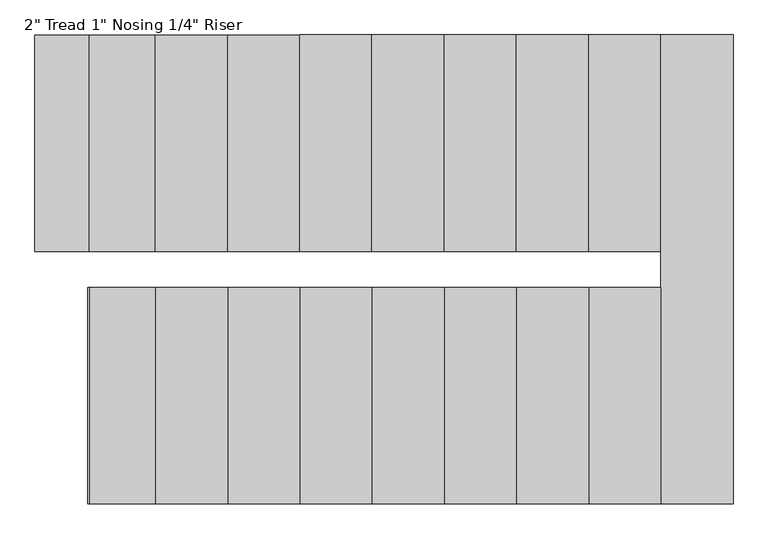
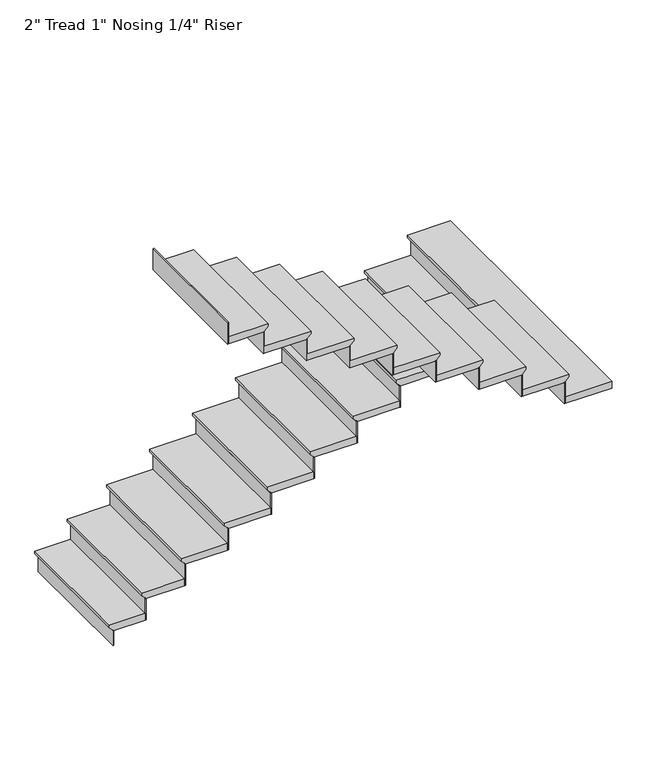
"""IFC4 building model written with IfcOpenShell, lengths in millimetres: stair flight geometry."""

from ifc_helpers import new_model, si_unit, origin, place, context, project, spatial, faceted_brep, source, transform, mapped, element, save


def stair_flight_4ae2a1ee(model_context):
    return source(origin(), model_context, "Body", "Brep", [
        faceted_brep([(8572.5, 8280.4, 12333.3710526), (8572.5, 8280.4, 12352.4210526), (8572.5, 9194.8, 12352.4210526), (8572.5, 9194.8, 12333.3710526), (8597.9, 8280.4, 12307.9710526), (8597.9, 9194.8, 12307.9710526), (8826.5, 8280.4, 12352.4210526), (8826.5, 9194.8, 12352.4210526), (8597.9, 9194.8, 12301.6210526), (8826.5, 9194.8, 12301.6210526), (8826.5, 8280.4, 12301.6210526), (8597.9, 8280.4, 12301.6210526)], [[[0, 1, 2, 3]], [[4, 0, 3, 5]], [[2, 1, 6, 7]], [[8, 9, 10, 11]], [[2, 7, 9, 8, 5, 3]], [[8, 11, 4, 5]], [[6, 1, 0, 4, 11, 10]], [[7, 6, 10, 9]]]),
        faceted_brep([(8597.9, 8280.4, 12301.6210526), (8597.9, 8280.4, 12192.0), (8604.25, 8280.4, 12192.0), (8604.25, 8280.4, 12301.6210526), (8597.9, 9194.8, 12301.6210526), (8604.25, 9194.8, 12301.6210526), (8604.25, 9194.8, 12192.0), (8597.9, 9194.8, 12192.0)], [[[0, 1, 2, 3]], [[4, 5, 6, 7]], [[1, 0, 4, 7]], [[2, 1, 7, 6]], [[3, 2, 6, 5]], [[0, 3, 5, 4]]]),
        faceted_brep([(8826.5, 8280.4, 12462.0421053), (8826.5, 8280.4, 12301.6210526), (8832.85, 8280.4, 12301.6210526), (8832.85, 8280.4, 12462.0421053), (8826.5, 9194.8, 12462.0421053), (8832.85, 9194.8, 12462.0421053), (8832.85, 9194.8, 12301.6210526), (8826.5, 9194.8, 12301.6210526)], [[[0, 1, 2, 3]], [[4, 5, 6, 7]], [[1, 0, 4, 7]], [[2, 1, 7, 6]], [[3, 2, 6, 5]], [[0, 3, 5, 4]]]),
        faceted_brep([(8801.1, 9194.8, 12512.8421053), (8801.1, 8280.4, 12512.8421053), (9105.9, 8280.4, 12512.8421053), (9105.9, 9194.8, 12512.8421053), (8826.5, 9194.8, 12462.0421053), (9105.9, 9194.8, 12462.0421053), (9105.9, 8280.4, 12462.0421053), (8826.5, 8280.4, 12462.0421053), (8826.5, 9194.8, 12468.3921053), (8801.1, 9194.8, 12493.7921053), (8826.5, 8280.4, 12468.3921053), (8801.1, 8280.4, 12493.7921053)], [[[0, 1, 2, 3]], [[4, 5, 6, 7]], [[0, 3, 5, 4, 8, 9]], [[4, 7, 10, 8]], [[2, 1, 11, 10, 7, 6]], [[3, 2, 6, 5]], [[11, 1, 0, 9]], [[10, 11, 9, 8]]]),
        faceted_brep([(9105.9, 8280.4, 12622.4631579), (9105.9, 8280.4, 12462.0421053), (9112.25, 8280.4, 12462.0421053), (9112.25, 8280.4, 12622.4631579), (9105.9, 9194.8, 12622.4631579), (9112.25, 9194.8, 12622.4631579), (9112.25, 9194.8, 12462.0421053), (9105.9, 9194.8, 12462.0421053)], [[[0, 1, 2, 3]], [[4, 5, 6, 7]], [[1, 0, 4, 7]], [[2, 1, 7, 6]], [[3, 2, 6, 5]], [[0, 3, 5, 4]]]),
        faceted_brep([(9080.5, 9194.8, 12673.2631579), (9080.5, 8280.4, 12673.2631579), (9410.7, 8280.4, 12673.2631579), (9410.7, 9194.8, 12673.2631579), (9105.9, 9194.8, 12622.4631579), (9410.7, 9194.8, 12622.4631579), (9410.7, 8280.4, 12622.4631579), (9105.9, 8280.4, 12622.4631579), (9105.9, 9194.8, 12628.8131579), (9080.5, 9194.8, 12654.2131579), (9105.9, 8280.4, 12628.8131579), (9080.5, 8280.4, 12654.2131579)], [[[0, 1, 2, 3]], [[4, 5, 6, 7]], [[0, 3, 5, 4, 8, 9]], [[4, 7, 10, 8]], [[2, 1, 11, 10, 7, 6]], [[3, 2, 6, 5]], [[11, 1, 0, 9]], [[10, 11, 9, 8]]]),
        faceted_brep([(9410.7, 8280.4, 12782.8842105), (9410.7, 8280.4, 12622.4631579), (9417.05, 8280.4, 12622.4631579), (9417.05, 8280.4, 12782.8842105), (9410.7, 9194.8, 12782.8842105), (9417.05, 9194.8, 12782.8842105), (9417.05, 9194.8, 12622.4631579), (9410.7, 9194.8, 12622.4631579)], [[[0, 1, 2, 3]], [[4, 5, 6, 7]], [[1, 0, 4, 7]], [[2, 1, 7, 6]], [[3, 2, 6, 5]], [[0, 3, 5, 4]]]),
        faceted_brep([(9385.3, 9194.8, 12833.6842105), (9385.3, 8280.4, 12833.6842105), (9715.5, 8280.4, 12833.6842105), (9715.5, 9194.8, 12833.6842105), (9410.7, 9194.8, 12782.8842105), (9715.5, 9194.8, 12782.8842105), (9715.5, 8280.4, 12782.8842105), (9410.7, 8280.4, 12782.8842105), (9410.7, 9194.8, 12789.2342105), (9385.3, 9194.8, 12814.6342105), (9410.7, 8280.4, 12789.2342105), (9385.3, 8280.4, 12814.6342105)], [[[0, 1, 2, 3]], [[4, 5, 6, 7]], [[0, 3, 5, 4, 8, 9]], [[4, 7, 10, 8]], [[2, 1, 11, 10, 7, 6]], [[3, 2, 6, 5]], [[11, 1, 0, 9]], [[10, 11, 9, 8]]]),
        faceted_brep([(9715.5, 8280.4, 12943.3052632), (9715.5, 8280.4, 12782.8842105), (9721.85, 8280.4, 12782.8842105), (9721.85, 8280.4, 12943.3052632), (9715.5, 9194.8, 12943.3052632), (9721.85, 9194.8, 12943.3052632), (9721.85, 9194.8, 12782.8842105), (9715.5, 9194.8, 12782.8842105)], [[[0, 1, 2, 3]], [[4, 5, 6, 7]], [[1, 0, 4, 7]], [[2, 1, 7, 6]], [[3, 2, 6, 5]], [[0, 3, 5, 4]]]),
        faceted_brep([(9690.1, 9194.8, 12994.1052632), (9690.1, 8280.4, 12994.1052632), (10020.3, 8280.4, 12994.1052632), (10020.3, 9194.8, 12994.1052632), (9715.5, 9194.8, 12943.3052632), (10020.3, 9194.8, 12943.3052632), (10020.3, 8280.4, 12943.3052632), (9715.5, 8280.4, 12943.3052632), (9715.5, 9194.8, 12949.6552632), (9690.1, 9194.8, 12975.0552632), (9715.5, 8280.4, 12949.6552632), (9690.1, 8280.4, 12975.0552632)], [[[0, 1, 2, 3]], [[4, 5, 6, 7]], [[0, 3, 5, 4, 8, 9]], [[4, 7, 10, 8]], [[2, 1, 11, 10, 7, 6]], [[3, 2, 6, 5]], [[11, 1, 0, 9]], [[10, 11, 9, 8]]]),
        faceted_brep([(10020.3, 8280.4, 13103.7263158), (10020.3, 8280.4, 12943.3052632), (10026.65, 8280.4, 12943.3052632), (10026.65, 8280.4, 13103.7263158), (10020.3, 9194.8, 13103.7263158), (10026.65, 9194.8, 13103.7263158), (10026.65, 9194.8, 12943.3052632), (10020.3, 9194.8, 12943.3052632)], [[[0, 1, 2, 3]], [[4, 5, 6, 7]], [[1, 0, 4, 7]], [[2, 1, 7, 6]], [[3, 2, 6, 5]], [[0, 3, 5, 4]]]),
        faceted_brep([(9994.9, 9194.8, 13154.5263158), (9994.9, 8280.4, 13154.5263158), (10325.1, 8280.4, 13154.5263158), (10325.1, 9194.8, 13154.5263158), (10020.3, 9194.8, 13103.7263158), (10325.1, 9194.8, 13103.7263158), (10325.1, 8280.4, 13103.7263158), (10020.3, 8280.4, 13103.7263158), (10020.3, 9194.8, 13110.0763158), (9994.9, 9194.8, 13135.4763158), (10020.3, 8280.4, 13110.0763158), (9994.9, 8280.4, 13135.4763158)], [[[0, 1, 2, 3]], [[4, 5, 6, 7]], [[0, 3, 5, 4, 8, 9]], [[4, 7, 10, 8]], [[2, 1, 11, 10, 7, 6]], [[3, 2, 6, 5]], [[11, 1, 0, 9]], [[10, 11, 9, 8]]]),
        faceted_brep([(10325.1, 8280.4, 13264.1473684), (10325.1, 8280.4, 13103.7263158), (10331.45, 8280.4, 13103.7263158), (10331.45, 8280.4, 13264.1473684), (10325.1, 9194.8, 13264.1473684), (10331.45, 9194.8, 13264.1473684), (10331.45, 9194.8, 13103.7263158), (10325.1, 9194.8, 13103.7263158)], [[[0, 1, 2, 3]], [[4, 5, 6, 7]], [[1, 0, 4, 7]], [[2, 1, 7, 6]], [[3, 2, 6, 5]], [[0, 3, 5, 4]]]),
        faceted_brep([(10299.7, 9194.8, 13314.9473684), (10299.7, 8280.4, 13314.9473684), (10629.9, 8280.4, 13314.9473684), (10629.9, 9194.8, 13314.9473684), (10325.1, 9194.8, 13264.1473684), (10629.9, 9194.8, 13264.1473684), (10629.9, 8280.4, 13264.1473684), (10325.1, 8280.4, 13264.1473684), (10325.1, 9194.8, 13270.4973684), (10299.7, 9194.8, 13295.8973684), (10325.1, 8280.4, 13270.4973684), (10299.7, 8280.4, 13295.8973684)], [[[0, 1, 2, 3]], [[4, 5, 6, 7]], [[0, 3, 5, 4, 8, 9]], [[4, 7, 10, 8]], [[2, 1, 11, 10, 7, 6]], [[3, 2, 6, 5]], [[11, 1, 0, 9]], [[10, 11, 9, 8]]]),
        faceted_brep([(10629.9, 8280.4, 13424.5684211), (10629.9, 8280.4, 13264.1473684), (10636.25, 8280.4, 13264.1473684), (10636.25, 8280.4, 13424.5684211), (10629.9, 9194.8, 13424.5684211), (10636.25, 9194.8, 13424.5684211), (10636.25, 9194.8, 13264.1473684), (10629.9, 9194.8, 13264.1473684)], [[[0, 1, 2, 3]], [[4, 5, 6, 7]], [[1, 0, 4, 7]], [[2, 1, 7, 6]], [[3, 2, 6, 5]], [[0, 3, 5, 4]]]),
        faceted_brep([(10604.5, 9194.8, 13475.3684211), (10604.5, 8280.4, 13475.3684211), (10934.7, 8280.4, 13475.3684211), (10934.7, 9194.8, 13475.3684211), (10629.9, 9194.8, 13424.5684211), (10934.7, 9194.8, 13424.5684211), (10934.7, 8280.4, 13424.5684211), (10629.9, 8280.4, 13424.5684211), (10629.9, 9194.8, 13430.9184211), (10604.5, 9194.8, 13456.3184211), (10629.9, 8280.4, 13430.9184211), (10604.5, 8280.4, 13456.3184211)], [[[0, 1, 2, 3]], [[4, 5, 6, 7]], [[0, 3, 5, 4, 8, 9]], [[4, 7, 10, 8]], [[2, 1, 11, 10, 7, 6]], [[3, 2, 6, 5]], [[11, 1, 0, 9]], [[10, 11, 9, 8]]]),
        faceted_brep([(10934.7, 8280.4, 13584.9894737), (10934.7, 8280.4, 13424.5684211), (10941.05, 8280.4, 13424.5684211), (10941.05, 8280.4, 13584.9894737), (10934.7, 9194.8, 13584.9894737), (10941.05, 9194.8, 13584.9894737), (10941.05, 9194.8, 13424.5684211), (10934.7, 9194.8, 13424.5684211)], [[[0, 1, 2, 3]], [[4, 5, 6, 7]], [[1, 0, 4, 7]], [[2, 1, 7, 6]], [[3, 2, 6, 5]], [[0, 3, 5, 4]]]),
        faceted_brep([(10909.3, 9194.8, 13635.7894737), (10909.3, 8280.4, 13635.7894737), (11239.5, 8280.4, 13635.7894737), (11239.5, 9194.8, 13635.7894737), (10934.7, 9194.8, 13584.9894737), (11239.5, 9194.8, 13584.9894737), (11239.5, 8280.4, 13584.9894737), (10934.7, 8280.4, 13584.9894737), (10934.7, 9194.8, 13591.3394737), (10909.3, 9194.8, 13616.7394737), (10934.7, 8280.4, 13591.3394737), (10909.3, 8280.4, 13616.7394737)], [[[0, 1, 2, 3]], [[4, 5, 6, 7]], [[0, 3, 5, 4, 8, 9]], [[4, 7, 10, 8]], [[2, 1, 11, 10, 7, 6]], [[3, 2, 6, 5]], [[11, 1, 0, 9]], [[10, 11, 9, 8]]]),
        faceted_brep([(11239.5, 8280.4, 13745.4105263), (11239.5, 8280.4, 13584.9894737), (11245.85, 8280.4, 13584.9894737), (11245.85, 8280.4, 13745.4105263), (11239.5, 9194.8, 13745.4105263), (11245.85, 9194.8, 13745.4105263), (11245.85, 9194.8, 13584.9894737), (11239.5, 9194.8, 13584.9894737)], [[[0, 1, 2, 3]], [[4, 5, 6, 7]], [[1, 0, 4, 7]], [[2, 1, 7, 6]], [[3, 2, 6, 5]], [[0, 3, 5, 4]]]),
        faceted_brep([(11188.7, 7213.6, 13796.2105263), (11518.9, 7213.6, 13796.2105263), (11518.9, 9194.8, 13796.2105263), (11214.1, 9194.8, 13796.2105263), (11214.1, 8128.0, 13796.2105263), (11188.7, 8128.0, 13796.2105263), (11518.9, 7213.6, 13745.4105263), (11188.7, 7213.6, 13745.4105263), (11188.7, 8128.0, 13745.4105263), (11214.1, 8128.0, 13745.4105263), (11214.1, 8280.4, 13745.4105263), (11239.5, 8280.4, 13745.4105263), (11239.5, 9194.8, 13745.4105263), (11518.9, 9194.8, 13745.4105263), (11239.5, 9194.8, 13751.7605263), (11214.1, 9194.8, 13777.1605263), (11239.5, 8280.4, 13751.7605263), (11214.1, 8280.4, 13777.1605263)], [[[0, 1, 2, 3, 4, 5]], [[6, 7, 8, 9, 10, 11, 12, 13]], [[1, 0, 7, 6]], [[2, 1, 6, 13]], [[3, 2, 13, 12, 14, 15]], [[12, 11, 16, 14]], [[11, 10, 17, 16]], [[4, 3, 15, 17, 10, 9]], [[5, 4, 9, 8]], [[0, 5, 8, 7]], [[15, 14, 16, 17]]]),
        faceted_brep([(11188.7, 8128.0, 13905.8315789), (11188.7, 8128.0, 13745.4105263), (11182.35, 8128.0, 13745.4105263), (11182.35, 8128.0, 13905.8315789), (11188.7, 7213.6, 13905.8315789), (11182.35, 7213.6, 13905.8315789), (11182.35, 7213.6, 13745.4105263), (11188.7, 7213.6, 13745.4105263)], [[[0, 1, 2, 3]], [[4, 5, 6, 7]], [[1, 0, 4, 7]], [[2, 1, 7, 6]], [[3, 2, 6, 5]], [[0, 3, 5, 4]]]),
        faceted_brep([(11214.1, 7213.6, 13956.6315789), (11214.1, 8128.0, 13956.6315789), (10883.9, 8128.0, 13956.6315789), (10883.9, 7213.6, 13956.6315789), (11188.7, 7213.6, 13905.8315789), (10883.9, 7213.6, 13905.8315789), (10883.9, 8128.0, 13905.8315789), (11188.7, 8128.0, 13905.8315789), (11188.7, 7213.6, 13912.1815789), (11214.1, 7213.6, 13937.5815789), (11188.7, 8128.0, 13912.1815789), (11214.1, 8128.0, 13937.5815789)], [[[0, 1, 2, 3]], [[4, 5, 6, 7]], [[0, 3, 5, 4, 8, 9]], [[4, 7, 10, 8]], [[2, 1, 11, 10, 7, 6]], [[3, 2, 6, 5]], [[11, 1, 0, 9]], [[10, 11, 9, 8]]]),
        faceted_brep([(10883.9, 8128.0, 14066.2526316), (10883.9, 8128.0, 13905.8315789), (10877.55, 8128.0, 13905.8315789), (10877.55, 8128.0, 14066.2526316), (10883.9, 7213.6, 14066.2526316), (10877.55, 7213.6, 14066.2526316), (10877.55, 7213.6, 13905.8315789), (10883.9, 7213.6, 13905.8315789)], [[[0, 1, 2, 3]], [[4, 5, 6, 7]], [[1, 0, 4, 7]], [[2, 1, 7, 6]], [[3, 2, 6, 5]], [[0, 3, 5, 4]]]),
        faceted_brep([(10909.3, 7213.6, 14117.0526316), (10909.3, 8128.0, 14117.0526316), (10579.1, 8128.0, 14117.0526316), (10579.1, 7213.6, 14117.0526316), (10883.9, 7213.6, 14066.2526316), (10579.1, 7213.6, 14066.2526316), (10579.1, 8128.0, 14066.2526316), (10883.9, 8128.0, 14066.2526316), (10883.9, 7213.6, 14072.6026316), (10909.3, 7213.6, 14098.0026316), (10883.9, 8128.0, 14072.6026316), (10909.3, 8128.0, 14098.0026316)], [[[0, 1, 2, 3]], [[4, 5, 6, 7]], [[0, 3, 5, 4, 8, 9]], [[4, 7, 10, 8]], [[2, 1, 11, 10, 7, 6]], [[3, 2, 6, 5]], [[11, 1, 0, 9]], [[10, 11, 9, 8]]]),
        faceted_brep([(10579.1, 8128.0, 14226.6736842), (10579.1, 8128.0, 14066.2526316), (10572.75, 8128.0, 14066.2526316), (10572.75, 8128.0, 14226.6736842), (10579.1, 7213.6, 14226.6736842), (10572.75, 7213.6, 14226.6736842), (10572.75, 7213.6, 14066.2526316), (10579.1, 7213.6, 14066.2526316)], [[[0, 1, 2, 3]], [[4, 5, 6, 7]], [[1, 0, 4, 7]], [[2, 1, 7, 6]], [[3, 2, 6, 5]], [[0, 3, 5, 4]]]),
        faceted_brep([(10604.5, 7213.6, 14277.4736842), (10604.5, 8128.0, 14277.4736842), (10274.3, 8128.0, 14277.4736842), (10274.3, 7213.6, 14277.4736842), (10579.1, 7213.6, 14226.6736842), (10274.3, 7213.6, 14226.6736842), (10274.3, 8128.0, 14226.6736842), (10579.1, 8128.0, 14226.6736842), (10579.1, 7213.6, 14233.0236842), (10604.5, 7213.6, 14258.4236842), (10579.1, 8128.0, 14233.0236842), (10604.5, 8128.0, 14258.4236842)], [[[0, 1, 2, 3]], [[4, 5, 6, 7]], [[0, 3, 5, 4, 8, 9]], [[4, 7, 10, 8]], [[2, 1, 11, 10, 7, 6]], [[3, 2, 6, 5]], [[11, 1, 0, 9]], [[10, 11, 9, 8]]]),
        faceted_brep([(10274.3, 8128.0, 14387.0947368), (10274.3, 8128.0, 14226.6736842), (10267.95, 8128.0, 14226.6736842), (10267.95, 8128.0, 14387.0947368), (10274.3, 7213.6, 14387.0947368), (10267.95, 7213.6, 14387.0947368), (10267.95, 7213.6, 14226.6736842), (10274.3, 7213.6, 14226.6736842)], [[[0, 1, 2, 3]], [[4, 5, 6, 7]], [[1, 0, 4, 7]], [[2, 1, 7, 6]], [[3, 2, 6, 5]], [[0, 3, 5, 4]]]),
        faceted_brep([(10299.7, 7213.6, 14437.8947368), (10299.7, 8128.0, 14437.8947368), (9969.5, 8128.0, 14437.8947368), (9969.5, 7213.6, 14437.8947368), (10274.3, 7213.6, 14387.0947368), (9969.5, 7213.6, 14387.0947368), (9969.5, 8128.0, 14387.0947368), (10274.3, 8128.0, 14387.0947368), (10274.3, 7213.6, 14393.4447368), (10299.7, 7213.6, 14418.8447368), (10274.3, 8128.0, 14393.4447368), (10299.7, 8128.0, 14418.8447368)], [[[0, 1, 2, 3]], [[4, 5, 6, 7]], [[0, 3, 5, 4, 8, 9]], [[4, 7, 10, 8]], [[2, 1, 11, 10, 7, 6]], [[3, 2, 6, 5]], [[11, 1, 0, 9]], [[10, 11, 9, 8]]]),
        faceted_brep([(9969.5, 8128.0, 14547.5157895), (9969.5, 8128.0, 14387.0947368), (9963.15, 8128.0, 14387.0947368), (9963.15, 8128.0, 14547.5157895), (9969.5, 7213.6, 14547.5157895), (9963.15, 7213.6, 14547.5157895), (9963.15, 7213.6, 14387.0947368), (9969.5, 7213.6, 14387.0947368)], [[[0, 1, 2, 3]], [[4, 5, 6, 7]], [[1, 0, 4, 7]], [[2, 1, 7, 6]], [[3, 2, 6, 5]], [[0, 3, 5, 4]]]),
        faceted_brep([(9994.9, 7213.6, 14598.3157895), (9994.9, 8128.0, 14598.3157895), (9664.7, 8128.0, 14598.3157895), (9664.7, 7213.6, 14598.3157895), (9969.5, 7213.6, 14547.5157895), (9664.7, 7213.6, 14547.5157895), (9664.7, 8128.0, 14547.5157895), (9969.5, 8128.0, 14547.5157895), (9969.5, 7213.6, 14553.8657895), (9994.9, 7213.6, 14579.2657895), (9969.5, 8128.0, 14553.8657895), (9994.9, 8128.0, 14579.2657895)], [[[0, 1, 2, 3]], [[4, 5, 6, 7]], [[0, 3, 5, 4, 8, 9]], [[4, 7, 10, 8]], [[2, 1, 11, 10, 7, 6]], [[3, 2, 6, 5]], [[11, 1, 0, 9]], [[10, 11, 9, 8]]]),
        faceted_brep([(9664.7, 8128.0, 14707.9368421), (9664.7, 8128.0, 14547.5157895), (9658.35, 8128.0, 14547.5157895), (9658.35, 8128.0, 14707.9368421), (9664.7, 7213.6, 14707.9368421), (9658.35, 7213.6, 14707.9368421), (9658.35, 7213.6, 14547.5157895), (9664.7, 7213.6, 14547.5157895)], [[[0, 1, 2, 3]], [[4, 5, 6, 7]], [[1, 0, 4, 7]], [[2, 1, 7, 6]], [[3, 2, 6, 5]], [[0, 3, 5, 4]]]),
        faceted_brep([(9690.1, 7213.6, 14758.7368421), (9690.1, 8128.0, 14758.7368421), (9359.9, 8128.0, 14758.7368421), (9359.9, 7213.6, 14758.7368421), (9664.7, 7213.6, 14707.9368421), (9359.9, 7213.6, 14707.9368421), (9359.9, 8128.0, 14707.9368421), (9664.7, 8128.0, 14707.9368421), (9664.7, 7213.6, 14714.2868421), (9690.1, 7213.6, 14739.6868421), (9664.7, 8128.0, 14714.2868421), (9690.1, 8128.0, 14739.6868421)], [[[0, 1, 2, 3]], [[4, 5, 6, 7]], [[0, 3, 5, 4, 8, 9]], [[4, 7, 10, 8]], [[2, 1, 11, 10, 7, 6]], [[3, 2, 6, 5]], [[11, 1, 0, 9]], [[10, 11, 9, 8]]]),
        faceted_brep([(9359.9, 8128.0, 14868.3578947), (9359.9, 8128.0, 14707.9368421), (9353.55, 8128.0, 14707.9368421), (9353.55, 8128.0, 14868.3578947), (9359.9, 7213.6, 14868.3578947), (9353.55, 7213.6, 14868.3578947), (9353.55, 7213.6, 14707.9368421), (9359.9, 7213.6, 14707.9368421)], [[[0, 1, 2, 3]], [[4, 5, 6, 7]], [[1, 0, 4, 7]], [[2, 1, 7, 6]], [[3, 2, 6, 5]], [[0, 3, 5, 4]]]),
        faceted_brep([(9385.3, 7213.6, 14919.1578947), (9385.3, 8128.0, 14919.1578947), (9055.1, 8128.0, 14919.1578947), (9055.1, 7213.6, 14919.1578947), (9359.9, 7213.6, 14868.3578947), (9055.1, 7213.6, 14868.3578947), (9055.1, 8128.0, 14868.3578947), (9359.9, 8128.0, 14868.3578947), (9359.9, 7213.6, 14874.7078947), (9385.3, 7213.6, 14900.1078947), (9359.9, 8128.0, 14874.7078947), (9385.3, 8128.0, 14900.1078947)], [[[0, 1, 2, 3]], [[4, 5, 6, 7]], [[0, 3, 5, 4, 8, 9]], [[4, 7, 10, 8]], [[2, 1, 11, 10, 7, 6]], [[3, 2, 6, 5]], [[11, 1, 0, 9]], [[10, 11, 9, 8]]]),
        faceted_brep([(9055.1, 8128.0, 15028.7789474), (9055.1, 8128.0, 14868.3578947), (9048.75, 8128.0, 14868.3578947), (9048.75, 8128.0, 15028.7789474), (9055.1, 7213.6, 15028.7789474), (9048.75, 7213.6, 15028.7789474), (9048.75, 7213.6, 14868.3578947), (9055.1, 7213.6, 14868.3578947)], [[[0, 1, 2, 3]], [[4, 5, 6, 7]], [[1, 0, 4, 7]], [[2, 1, 7, 6]], [[3, 2, 6, 5]], [[0, 3, 5, 4]]]),
        faceted_brep([(8801.1, 8128.0, 15189.2), (8801.1, 8128.0, 15028.7789474), (8794.75, 8128.0, 15028.7789474), (8794.75, 8128.0, 15189.2), (8801.1, 7213.6, 15189.2), (8794.75, 7213.6, 15189.2), (8794.75, 7213.6, 15028.7789474), (8801.1, 7213.6, 15028.7789474)], [[[0, 1, 2, 3]], [[4, 5, 6, 7]], [[1, 0, 4, 7]], [[2, 1, 7, 6]], [[3, 2, 6, 5]], [[0, 3, 5, 4]]]),
        faceted_brep([(9080.5, 7213.6, 15079.5789474), (9080.5, 8128.0, 15079.5789474), (8801.1, 8128.0, 15079.5789474), (8801.1, 7213.6, 15079.5789474), (9055.1, 7213.6, 15028.7789474), (8801.1, 7213.6, 15028.7789474), (8801.1, 8128.0, 15028.7789474), (9055.1, 8128.0, 15028.7789474), (9055.1, 7213.6, 15035.1289474), (9080.5, 7213.6, 15060.5289474), (9055.1, 8128.0, 15035.1289474), (9080.5, 8128.0, 15060.5289474)], [[[0, 1, 2, 3]], [[4, 5, 6, 7]], [[0, 3, 5, 4, 8, 9]], [[4, 7, 10, 8]], [[2, 1, 11, 10, 7, 6]], [[3, 2, 6, 5]], [[11, 1, 0, 9]], [[10, 11, 9, 8]]]),
    ])


if __name__ == "__main__":
    model = new_model("IFC4")
    model_context = context("Model", 3, world=origin())
    ifc_project = project(units=[si_unit("LENGTHUNIT", "METRE", prefix="MILLI")], contexts=[model_context])
    site = spatial("IfcSite", under=ifc_project)
    building = spatial("IfcBuilding", under=site)
    placement = place(None, origin())
    stair_flight_shape = stair_flight_4ae2a1ee(model_context)
    element("IfcStairFlight", 1, ObjectType="2\" Tread 1\" Nosing 1/4\" Riser", at=placement, inside=building, context=model_context, shape_type="MappedRepresentation", body=[
        mapped(stair_flight_shape, transform((0.0, 0.0, 0.0), x_axis=(1.0, 0.0, 0.0), y_axis=(0.0, 1.0, 0.0), z_axis=(0.0, 0.0, 1.0))),
    ])
    save(model, "model.ifc")
